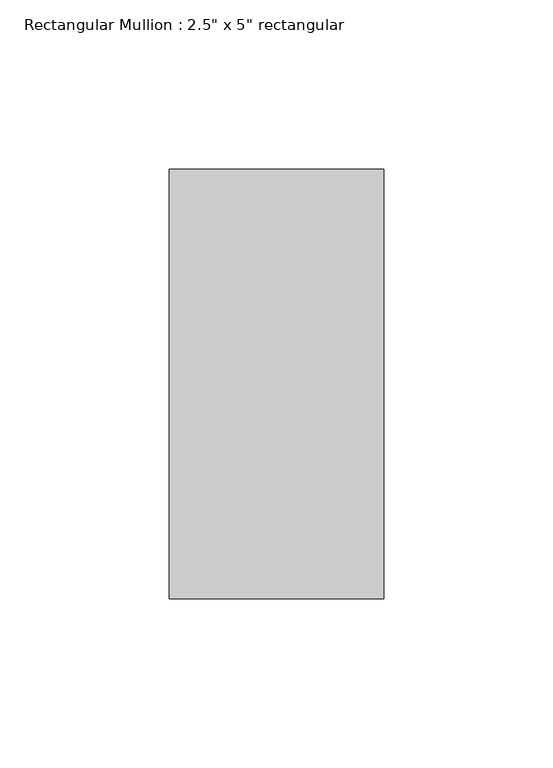
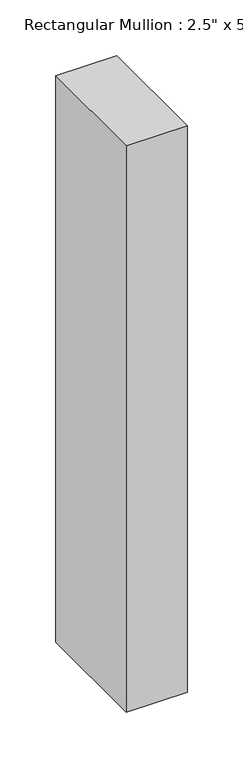
"""IFC4 building model written with IfcOpenShell, lengths in millimetres: member geometry."""

from ifc_helpers import new_model, si_unit, frame, origin, place, context, project, spatial, polyline, outline, extrude, source, transform, mapped, element, save


def member_081e0693(model_context):
    return source(origin(), model_context, "Body", "SweptSolid", [
        extrude(outline(polyline([(0.0, 63.5), (0.0, -63.5), (-63.5, -63.5), (-63.5, 63.5), (0.0, 63.5)])), frame((0.0, 0.0, -622.3), z_axis=(0.0, 0.0, 1.0), x_axis=(1.0, 0.0, 0.0)), (0.0, 0.0, 1.0), 622.3),
    ])


if __name__ == "__main__":
    model = new_model("IFC4")
    model_context = context("Model", 3, world=origin())
    ifc_project = project(units=[si_unit("LENGTHUNIT", "METRE", prefix="MILLI")], contexts=[model_context])
    site = spatial("IfcSite", under=ifc_project)
    building = spatial("IfcBuilding", under=site)
    placement = place(None, origin())
    member_shape = member_081e0693(model_context)
    element("IfcMember", 1, ObjectType="Rectangular Mullion : 2.5\" x 5\" rectangular", at=placement, inside=building, context=model_context, shape_type="MappedRepresentation", body=[
        mapped(member_shape, transform((0.0, 0.0, 0.0), x_axis=(1.0, 0.0, 0.0), y_axis=(0.0, 1.0, 0.0), z_axis=(0.0, 0.0, 1.0))),
    ])
    save(model, "model.ifc")

# Revit data of these elements
# Type "Rectangular Mullion : 2.5\" x 5\" rectangular"
#   built-in parameter 1007304 = 0.416667 (stored number, unit not read)
#   built-in parameter 1007301 = 0.104167 (stored number, unit not read)
#   built-in parameter 1007300 = 0.104167 (stored number, unit not read)
# Element 1 (IfcMember, "Rectangular Mullion : 2.5\" x 5\" rectangular")
#   Materials on its faces: "Rectangle 1 sq"
# Materials
#   "Rectangle 1 sq": class "Generic", colour RGB 120 120 120, transparency 0, Cost = 0
